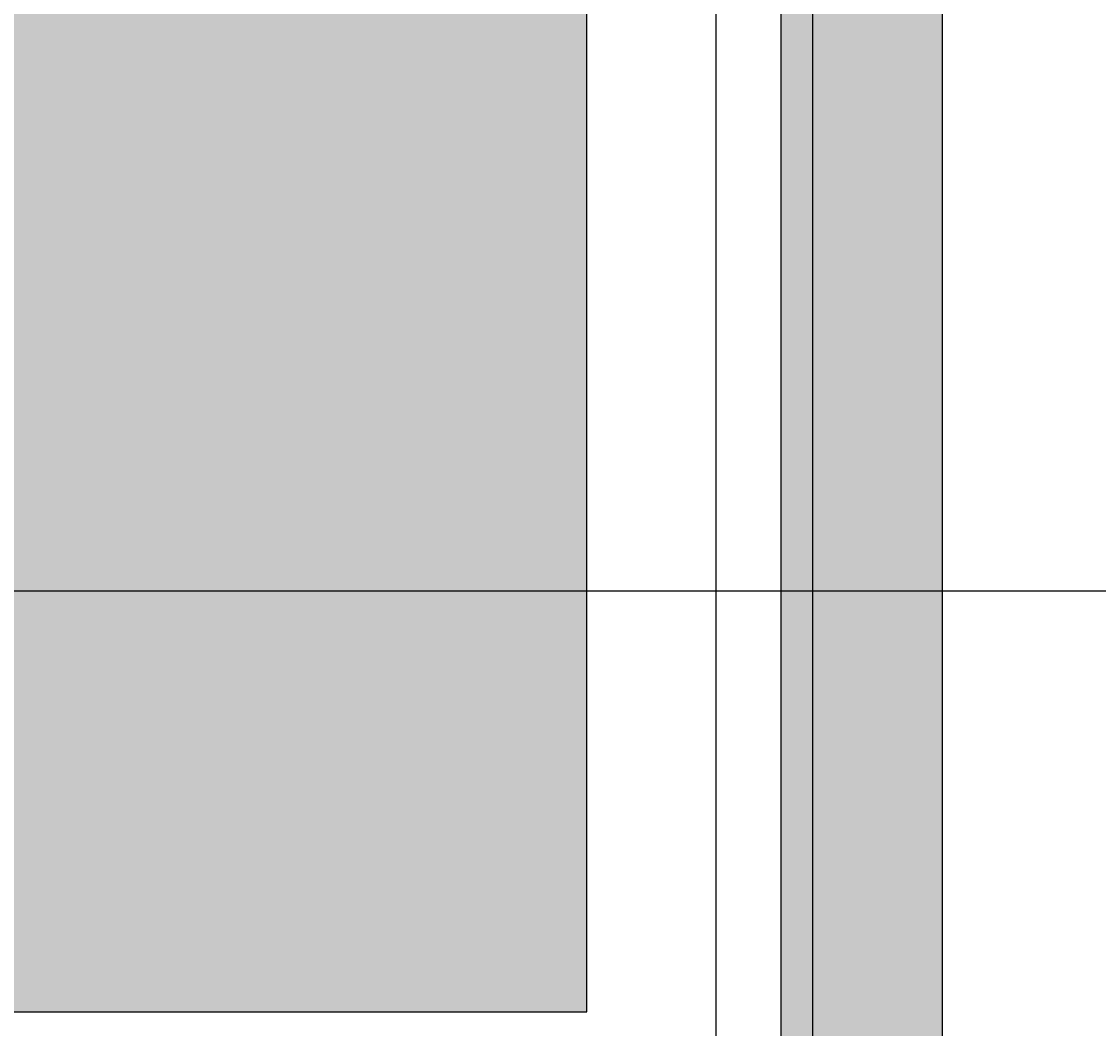
# Model space of a CAD drawing. Units: inches. Extents: x -301 to 715, y -607 to 364.
# Tile 23 of 141: x -16 to 18, y -453 to -422. Entities that reach past the tile are written whole.
import ezdxf

# ---------------------------------------------------------------- set-up
doc = ezdxf.new("R2010")
doc.units = ezdxf.units.IN
doc.header["$MEASUREMENT"] = 0
for name, color, linetype, lineweight in [('A-ANNO-DIMS', 2, 'Continuous', 18), ('A-DOOR', 4, 'Continuous', 25), ('A-SECT-PATT', 8, 'Continuous', 13)]:
    doc.layers.add(name, color=color, linetype=linetype, lineweight=lineweight)
doc.styles.get("Standard").update_dxf_attribs({"font": 'arial.ttf'})
doc.dimstyles.get("Standard").update_dxf_attribs({"dimtxt": 0.18, "dimasz": 0.18, "dimexe": 0.18, "dimexo": 0.0625, "dimgap": 0.09, "dimtad": 0, "dimtih": 1, "dimtoh": 1, "dimdec": 1, "dimzin": 0, "dimdsep": 46, "dimlunit": 4, "dimtxsty": 'Standard', "dimcen": 0.09, "dimclrd": 3, "dimclre": 4, "dimclrt": 6, "dimadec": 0, "dimazin": 0, "dimtfac": 1, "dimtdec": 1, "dimtofl": 0, "dimtmove": 0, "dimatfit": 3, "dimfxl": 1, "dimtfill": 2, "dimtfillclr": 51, "dimtolj": 1, "dimtzin": 0, "dimarcsym": 0})

# ---------------------------------------------------------------- blocks, each defined once
blk = doc.blocks.new('*U75')
blk.add_lwpolyline([(3.124, 0.013), (0.124, 0.013), (0.124, 72.013), (40.124, 72.013), (40.124, 0.013), (37.124, 0.013)])
for points in [[(37.124, 68.99), (37.124, 0.013), (3.124, 0.013), (3.124, 68.99)], [(33.124, 6.013), (33.124, 62.99), (7.124, 62.99), (7.124, 6.013)]]:
    blk.add_lwpolyline(points, close=True)
blk = doc.blocks.new('*D176')
at = {"layer": 'A-ANNO-DIMS', "color": 4, "lineweight": -2, "transparency": 16777216}
for p, q in [((148.28, -324.477), (215.605, -324.477)), ((-15.22, -540.477), (215.605, -540.477))]:
    blk.add_line(p, q, dxfattribs=at)
at = {"layer": 'A-ANNO-DIMS', "color": 3, "lineweight": -2, "transparency": 16777216}
for p, q in [((215.425, -324.657), (215.425, -432.296)), ((215.425, -540.297), (215.425, -432.659))]:
    blk.add_line(p, q, dxfattribs=at)
at = {"layer": 'A-ANNO-DIMS', "color": 3, "transparency": 16777216}
for points in [[(215.395, -324.657), (215.455, -324.657), (215.425, -324.477)], [(215.395, -540.297), (215.455, -540.297), (215.425, -540.477)]]:
    blk.add_solid(points, dxfattribs=at)
at = {"layer": 'Defpoints', "color": 0, "transparency": 16777216}
for p in [(148.218, -324.477), (-15.282, -540.477), (215.425, -540.477)]:
    blk.add_point(p, dxfattribs=at)
at = {"layer": 'A-ANNO-DIMS', "color": 6, "transparency": 16777216, "insert": (215.425, -432.477), "char_height": 0.18, "attachment_point": 5, "bg_fill": 1, "box_fill_scale": 1.25, "bg_fill_color": 51, "bg_fill_transparency": 0}
blk.add_mtext('\\A1;18\'-0"', dxfattribs=at)
blk = doc.blocks.new('*D181')
at = {"layer": 'A-ANNO-DIMS', "color": 4, "lineweight": -2, "transparency": 16777216}
for p, q in [((48.468, -433.54), (48.468, -573.809)), ((12.718, -463.54), (12.718, -573.809))]:
    blk.add_line(p, q, dxfattribs=at)
at = {"layer": 'A-ANNO-DIMS', "color": 3, "lineweight": -2, "transparency": 16777216}
for p, q in [((12.898, -573.629), (30.264, -573.629)), ((48.288, -573.629), (30.922, -573.629))]:
    blk.add_line(p, q, dxfattribs=at)
at = {"layer": 'A-ANNO-DIMS', "color": 3, "transparency": 16777216}
for points in [[(12.898, -573.599), (12.898, -573.659), (12.718, -573.629)], [(48.288, -573.599), (48.288, -573.659), (48.468, -573.629)]]:
    blk.add_solid(points, dxfattribs=at)
at = {"layer": 'Defpoints', "color": 0, "transparency": 16777216}
for p in [(48.468, -433.477), (12.718, -463.477), (48.468, -573.629)]:
    blk.add_point(p, dxfattribs=at)
at = {"layer": 'A-ANNO-DIMS', "color": 6, "transparency": 16777216, "insert": (30.593, -573.629), "char_height": 0.18, "attachment_point": 5, "bg_fill": 1, "box_fill_scale": 1.25, "bg_fill_color": 51, "bg_fill_transparency": 0}
blk.add_mtext('\\A1;3\'-0"', dxfattribs=at)
blk = doc.blocks.new('*D187')
at = {"layer": 'A-ANNO-DIMS', "color": 4, "lineweight": -2, "transparency": 16777216}
for p, q in [((139.674, -385.477), (-266.112, -385.477)), ((143.155, -439.477), (-266.112, -439.477))]:
    blk.add_line(p, q, dxfattribs=at)
at = {"layer": 'A-ANNO-DIMS', "color": 3, "lineweight": -2, "transparency": 16777216}
for p, q in [((-265.932, -385.657), (-265.932, -412.296)), ((-265.932, -439.297), (-265.932, -412.659))]:
    blk.add_line(p, q, dxfattribs=at)
at = {"layer": 'A-ANNO-DIMS', "color": 3, "transparency": 16777216}
for points in [[(-265.962, -385.657), (-265.902, -385.657), (-265.932, -385.477)], [(-265.962, -439.297), (-265.902, -439.297), (-265.932, -439.477)]]:
    blk.add_solid(points, dxfattribs=at)
at = {"layer": 'Defpoints', "color": 0, "transparency": 16777216}
for p in [(-265.932, -385.477), (139.737, -385.477), (143.218, -439.477)]:
    blk.add_point(p, dxfattribs=at)
at = {"layer": 'A-ANNO-DIMS', "color": 6, "transparency": 16777216, "insert": (-265.932, -412.477), "char_height": 0.18, "attachment_point": 5, "bg_fill": 1, "box_fill_scale": 1.25, "bg_fill_color": 51, "bg_fill_transparency": 0}
blk.add_mtext('\\A1;4\'-6"', dxfattribs=at)

msp = doc.modelspace()

# ---------------------------------------------------------------- hatches: boundary and pattern name
at = {"layer": 'A-SECT-PATT'}
h = msp.add_hatch(color=256, dxfattribs=at)
h.dxf.hatch_style = 1
h.paths.add_polyline_path([(-138.282, -385.477), (-138.282, -433.477), (-87.981, -433.477), (-87.981, -385.477)])
h.paths.add_polyline_path([(-92.981, -390.477), (-92.981, -428.477), (-133.282, -428.477), (-133.282, -390.477)], flags=16)
h.paths.add_polyline_path([(-35.282, -385.477), (-35.282, -463.477), (12.718, -463.477), (12.718, -385.477)])
h.paths.add_polyline_path([(-30.282, -390.477), (7.718, -390.477), (7.718, -458.477), (-30.282, -458.477)], flags=16)
h.paths.add_polyline_path([(48.468, -385.477), (48.468, -433.477), (98.468, -433.477), (98.468, -385.477)])
h.paths.add_polyline_path([(93.468, -390.477), (93.468, -428.477), (53.468, -428.477), (53.468, -390.477)], flags=16)
h = msp.add_hatch(color=256, dxfattribs=at)
h.dxf.hatch_style = 1
h.paths.add_polyline_path([(-24.297, -452.509), (1.703, -452.509), (1.703, -395.532), (-24.297, -395.532)])

# ---------------------------------------------------------------- linework, layer by layer
at = {"layer": 'A-DOOR'}
for points in [[(-35.282, -385.477), (12.718, -385.477), (12.718, -463.477), (-35.282, -463.477)], [(-30.282, -390.477), (7.718, -390.477), (7.718, -458.477), (-30.282, -458.477)]]:
    msp.add_lwpolyline(points, close=True, dxfattribs=at)

# ---------------------------------------------------------------- block references
msp.add_blockref('*U75', (-31.421, -458.522), dxfattribs=at)

# ---------------------------------------------------------------- dimensions: what is measured, and where the dimension line sits
at = {"layer": 'A-ANNO-DIMS'}
for base, p1, p2, picture, middle in [((215.425, -540.477), (148.218, -324.477), (-15.282, -540.477), '*D176', (215.425, -432.477)), ((-265.932, -385.477), (143.218, -439.477), (139.737, -385.477), '*D187', (-265.932, -412.477))]:
    dim = msp.add_linear_dim(base=base, p1=p1, p2=p2, angle=90, dimstyle='Standard', override={"dimdec": 1, "dimlfac": 1, "dimrnd": 0, "dimzin": 1, "dimdsep": 46, "dimlunit": 4, "dimfrac": 2}, dxfattribs=at)
    dim.commit()
    dim.dimension.update_dxf_attribs({"geometry": picture, "text_midpoint": middle})
dim = msp.add_linear_dim(base=(48.467984, -573.628877), p1=(12.717984, -463.47741), p2=(48.467984, -433.47741), dimstyle='Standard', override={"dimdec": 1, "dimlfac": 1, "dimrnd": 0, "dimzin": 1, "dimdsep": 46, "dimlunit": 4, "dimfrac": 2}, dxfattribs=at)
dim.commit()
dim.dimension.update_dxf_attribs({"geometry": '*D181', "text_midpoint": (30.592984, -573.628877)})

doc.saveas('drawing.dxf')
